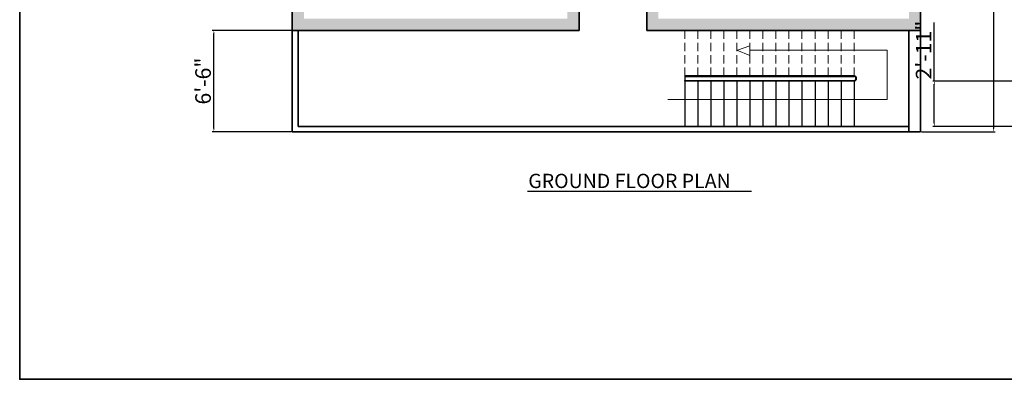
# Model space of a CAD drawing. Units: inches. Extents: x 1266 to 2869, y -408 to 3241.
# Tile 1 of 11: x 1266 to 2023, y 987 to 1264. Entities that reach past the tile are written whole.
import ezdxf

# ---------------------------------------------------------------- set-up
doc = ezdxf.new("R2010")
doc.units = ezdxf.units.IN
doc.linetypes.add('DASHED2', pattern=[9.525, 6.35, -3.175])
for name, color, linetype, lineweight in [('A-ANNO-DIMS', 2, 'Continuous', 18), ('A-ANNO-SYMB', 7, 'Continuous', 18), ('A-ANNO-TITL', 7, 'Continuous', 25), ('A-ANNO-TTLB', 7, 'Continuous', 35), ('A-FLOR-STRS', 7, 'Continuous', 25), ('A-FLOR-STRS-OVHD', 8, 'DASHED2', 18), ('A-WALL', 7, 'Continuous', 35), ('A-WALL-PATT', 251, 'Continuous', 13)]:
    doc.layers.add(name, color=color, linetype=linetype, lineweight=lineweight)
doc.styles.get("Standard").update_dxf_attribs({"font": 'arial.ttf'})
doc.dimstyles.new('ISO-25', dxfattribs={"dimtxt": 12, "dimasz": 2.5, "dimexe": 1.25, "dimexo": 0.625, "dimtad": 1, "dimdec": 0, "dimlunit": 3, "dimtxsty": 'Standard', "dimcen": 2.5, "dimadec": 0, "dimazin": 0, "dimtfac": 1, "dimtdec": 0, "dimtmove": 0, "dimatfit": 3, "dimfxl": 1, "dimarcsym": 0})

# ---------------------------------------------------------------- blocks, each defined once
blk = doc.blocks.new('*D3')
at = {"layer": 'A-ANNO-DIMS', "color": 0, "lineweight": -2, "transparency": 16777216}
for p, q in [((1959.32, 2278.35), (2016.1, 2278.35)), ((2014.85, 2275.85), (2014.85, 1179.85)), ((1959.32, 1177.35), (2016.1, 1177.35))]:
    blk.add_line(p, q, dxfattribs=at)
at = {"layer": 'A-ANNO-DIMS', "color": 0, "transparency": 16777216}
for points in [[(2014.43, 2275.85), (2015.27, 2275.85), (2014.85, 2278.35)], [(2014.43, 1179.85), (2015.27, 1179.85), (2014.85, 1177.35)]]:
    blk.add_solid(points, dxfattribs=at)
at = {"layer": 'Defpoints', "color": 0, "transparency": 16777216}
for p in [(1958.69, 2278.35), (1958.69, 1177.35), (2014.85, 1177.35)]:
    blk.add_point(p, dxfattribs=at)
at = {"layer": 'A-ANNO-DIMS', "color": 0, "transparency": 16777216, "insert": (2008.1, 1727.85), "char_height": 12, "attachment_point": 5, "rotation": 90}
blk.add_mtext('91\'-9"', dxfattribs=at)
blk = doc.blocks.new('STAIR-PATH-RETURN')
for p, q in [((53.2, 38.03), (63.2, 33.87)), ((53.5, 38.03), (53.2, 38.03)), ((63.2, 41.3), (53.5, 38.03)), ((63.2, 33.87), (63.2, 41.3)), ((168.66, 38.03), (63.2, 38.03)), ((168.66, 0), (168.66, 38.03)), ((0, 0), (168.66, 0))]:
    blk.add_line(p, q)
blk = doc.blocks.new('*D84')
at = {"layer": 'A-ANNO-DIMS', "color": 0, "lineweight": -2, "transparency": 16777216}
for p, q in [((1475.07, 1255.35), (1414.24, 1255.35)), ((1415.49, 1179.85), (1415.49, 1252.85)), ((1475.07, 1177.35), (1414.24, 1177.35))]:
    blk.add_line(p, q, dxfattribs=at)
at = {"layer": 'A-ANNO-DIMS', "color": 0, "transparency": 16777216}
for points in [[(1415.08, 1252.85), (1415.91, 1252.85), (1415.49, 1255.35)], [(1415.08, 1179.85), (1415.91, 1179.85), (1415.49, 1177.35)]]:
    blk.add_solid(points, dxfattribs=at)
at = {"layer": 'Defpoints', "color": 0, "transparency": 16777216}
for p in [(1415.49, 1255.35), (1475.69, 1255.35), (1475.69, 1177.35)]:
    blk.add_point(p, dxfattribs=at)
at = {"layer": 'A-ANNO-DIMS', "color": 0, "transparency": 16777216, "insert": (1408.74, 1216.35), "char_height": 12, "attachment_point": 5, "rotation": 90}
blk.add_mtext('6\'-6"', dxfattribs=at)
blk = doc.blocks.new('*D87')
at = {"layer": 'A-ANNO-DIMS', "color": 0, "lineweight": -2, "transparency": 16777216}
for p, q in [((1969.26, 1216.35), (1969.26, 1261.52)), ((2453.69, 1216.35), (1968.01, 1216.35)), ((1969.26, 1183.9), (1969.26, 1213.85)), ((2453.69, 1181.4), (1968.01, 1181.4))]:
    blk.add_line(p, q, dxfattribs=at)
at = {"layer": 'A-ANNO-DIMS', "color": 0, "transparency": 16777216}
for points in [[(1968.84, 1213.85), (1969.68, 1213.85), (1969.26, 1216.35)], [(1968.84, 1183.9), (1969.68, 1183.9), (1969.26, 1181.4)]]:
    blk.add_solid(points, dxfattribs=at)
at = {"layer": 'Defpoints', "color": 0, "transparency": 16777216}
for p in [(1969.26, 1216.35), (2454.31, 1216.35), (2454.31, 1181.4)]:
    blk.add_point(p, dxfattribs=at)
at = {"layer": 'A-ANNO-DIMS', "color": 0, "transparency": 16777216, "insert": (1962.61, 1240.19), "char_height": 12, "attachment_point": 5, "rotation": 90}
blk.add_mtext('2\'-11"', dxfattribs=at)

msp = doc.modelspace()

# ---------------------------------------------------------------- hatches: boundary and pattern name
at = {"layer": 'A-WALL-PATT'}
h = msp.add_hatch(color=256, dxfattribs=at)
h.dxf.hatch_style = 1
h.paths.add_polyline_path([(1484.69, 2269.35), (1562.69, 2269.35), (1562.69, 2149.35), (1558.42, 2149.35), (1558.42, 2144.85), (1567.19, 2144.85), (1573.23, 2144.85), (1573.23, 2146.74), (1573.23, 2149.35), (1567.19, 2149.35), (1567.19, 2269.35), (1597.45, 2269.35), (1597.45, 2273.85), (1597.45, 2278.35), (1475.69, 2278.35), (1475.69, 2234.52), (1484.69, 2234.52)])
h.paths.add_polyline_path([(1873.25, 2278.35), (1748.19, 2278.35), (1696.19, 2278.35), (1657.45, 2278.35), (1657.45, 2269.35), (1687.19, 2269.35), (1687.19, 2149.35), (1651.94, 2149.35), (1651.94, 2144.85), (1687.19, 2144.85), (1687.19, 2133.61), (1696.19, 2133.61), (1696.19, 2269.35), (1748.19, 2269.35), (1748.19, 2234.52), (1757.19, 2234.52), (1757.19, 2269.35), (1835.19, 2269.35), (1835.19, 2149.35), (1827.33, 2149.35), (1827.33, 2144.85), (1843.74, 2144.85), (1843.74, 2149.35), (1839.69, 2149.35), (1839.69, 2269.35), (1873.25, 2269.35), (1873.25, 2273.85)])
h.paths.add_polyline_path([(1958.69, 2278.35), (1933.25, 2278.35), (1933.25, 2269.35), (1949.69, 2269.35), (1949.69, 2149.35), (1912.22, 2149.35), (1912.22, 2144.85), (1949.69, 2144.85), (1949.69, 2133.61), (1958.69, 2133.61)])
h.paths.add_polyline_path([(1883.69, 2144.85), (1889.08, 2144.85), (1889.08, 2149.35), (1875.58, 2149.35), (1875.58, 2144.85), (1879.19, 2144.85), (1879.19, 2092.35), (1949.69, 2092.35), (1949.69, 2086.89), (1949.69, 2024.85), (1933.25, 2024.85), (1933.25, 2015.85), (1949.69, 2015.85), (1949.69, 1895.85), (1912.45, 1895.85), (1912.45, 1891.35), (1949.69, 1891.35), (1949.69, 1880.11), (1958.69, 1880.11), (1958.69, 2086.89), (1958.69, 2109.61), (1949.69, 2109.61), (1949.69, 2096.85), (1883.69, 2096.85)])
h.paths.add_polyline_path([(1757.19, 2198.52), (1748.19, 2198.52), (1748.19, 2086.89), (1757.19, 2086.89), (1757.19, 2144.85), (1793.55, 2144.85), (1793.55, 2149.35), (1757.19, 2149.35)])
h.paths.add_polyline_path([(1696.19, 2109.61), (1687.19, 2109.61), (1687.19, 2096.85), (1621.19, 2096.85), (1621.19, 2144.85), (1627.24, 2144.85), (1627.24, 2149.35), (1616.69, 2149.35), (1610.35, 2149.35), (1610.35, 2144.85), (1616.69, 2144.85), (1616.69, 2092.35), (1687.19, 2092.35), (1687.19, 2086.89), (1696.19, 2086.89)], flags=17)
h.paths.add_polyline_path([(1484.69, 2144.85), (1520.8, 2144.85), (1520.8, 2149.35), (1484.69, 2149.35), (1484.69, 2198.52), (1475.69, 2198.52), (1475.69, 1981.02), (1484.69, 1981.02), (1484.69, 2015.85), (1687.19, 2015.85), (1687.19, 1895.85), (1650.13, 1895.85), (1650.13, 1891.35), (1687.19, 1891.35), (1687.19, 1880.11), (1696.19, 1880.11), (1696.19, 2035.62), (1687.19, 2035.62), (1687.19, 2024.85), (1484.69, 2024.85)])
h.paths.add_polyline_path([(1484.69, 1691.52), (1475.69, 1691.52), (1475.69, 1474.02), (1484.69, 1474.02)])
h.paths.add_polyline_path([(1518.03, 1895.85), (1484.69, 1895.85), (1484.69, 1945.02), (1475.69, 1945.02), (1475.69, 1727.52), (1484.69, 1727.52), (1484.69, 1762.35), (1687.19, 1762.35), (1687.19, 1642.35), (1651.94, 1642.35), (1651.94, 1637.85), (1687.19, 1637.85), (1687.19, 1589.85), (1621.19, 1589.85), (1621.19, 1637.85), (1627.19, 1637.85), (1627.19, 1642.35), (1610.89, 1642.35), (1610.89, 1637.85), (1616.69, 1637.85), (1616.69, 1585.35), (1687.19, 1585.35), (1687.19, 1579.45), (1696.19, 1579.45), (1696.19, 1779.84), (1687.19, 1779.84), (1687.19, 1771.35), (1484.69, 1771.35), (1484.69, 1891.35), (1518.03, 1891.35)])
h.paths.add_polyline_path([(1567.19, 2015.85), (1562.69, 2015.85), (1562.69, 1895.85), (1555.64, 1895.85), (1555.64, 1891.35), (1570.46, 1891.35), (1570.46, 1895.85), (1567.19, 1895.85)], flags=17)
h.paths.add_polyline_path([(1625.43, 1895.85), (1607.58, 1895.85), (1607.58, 1891.35), (1616.69, 1891.35), (1616.69, 1838.85), (1687.19, 1838.85), (1687.19, 1831.11), (1696.19, 1831.11), (1696.19, 1856.11), (1687.19, 1856.11), (1687.19, 1843.35), (1621.19, 1843.35), (1621.19, 1891.35), (1625.43, 1891.35)], flags=17)
h.paths.add_polyline_path([(1567.19, 1762.35), (1562.69, 1762.35), (1562.69, 1642.35), (1558.42, 1642.35), (1558.42, 1637.85), (1573.23, 1637.85), (1573.23, 1642.35), (1567.19, 1642.35)], flags=17)
h.paths.add_polyline_path([(1520.8, 1642.35), (1484.69, 1642.35), (1484.69, 1637.85), (1520.8, 1637.85)], flags=17)
h.paths.add_polyline_path([(1687.19, 1517.85), (1484.69, 1517.85), (1484.69, 1508.85), (1562.69, 1508.85), (1562.69, 1388.85), (1567.19, 1388.85), (1567.19, 1508.85), (1687.19, 1508.85)])
h.paths.add_polyline_path([(1696.19, 1528.18), (1687.19, 1528.18), (1687.19, 1323.21), (1696.19, 1323.21)])
h.paths.add_polyline_path([(1696.19, 1271.94), (1687.19, 1271.94), (1687.19, 1264.35), (1484.69, 1264.35), (1484.69, 1283.77), (1480.19, 1283.77), (1475.69, 1283.77), (1475.69, 1255.35), (1480.19, 1255.35), (1696.19, 1255.35)])
h.paths.add_polyline_path([(1484.69, 1438.02), (1475.69, 1438.02), (1475.69, 1319.77), (1484.69, 1319.77)])
h.paths.add_polyline_path([(1873.25, 1513.35), (1873.25, 1517.85), (1757.19, 1517.85), (1757.19, 1528.62), (1748.19, 1528.62), (1748.19, 1474.02), (1757.19, 1474.02), (1757.19, 1508.85), (1835.19, 1508.85), (1835.19, 1388.85), (1827.33, 1388.85), (1827.33, 1384.35), (1843.74, 1384.35), (1843.74, 1388.85), (1839.69, 1388.85), (1839.69, 1508.85), (1873.25, 1508.85)])
h.paths.add_polyline_path([(1958.69, 1602.61), (1949.69, 1602.61), (1949.69, 1517.85), (1933.25, 1517.85), (1933.25, 1508.85), (1949.69, 1508.85), (1949.69, 1388.85), (1912.22, 1388.85), (1912.22, 1384.35), (1949.69, 1384.35), (1949.69, 1373.11), (1958.69, 1373.11)])
h.paths.add_polyline_path([(1958.69, 1349.11), (1949.69, 1349.11), (1949.69, 1336.35), (1883.69, 1336.35), (1883.69, 1384.35), (1889.08, 1384.35), (1889.08, 1388.85), (1875.58, 1388.85), (1875.58, 1384.35), (1879.19, 1384.35), (1879.19, 1331.85), (1949.69, 1331.85), (1949.69, 1315.59), (1958.69, 1315.59)])
h.paths.add_polyline_path([(1958.69, 1279.59), (1954.19, 1279.59), (1949.69, 1279.59), (1949.69, 1264.35), (1757.19, 1264.35), (1757.19, 1275.12), (1748.19, 1275.12), (1748.19, 1255.35), (1958.69, 1255.35)])
h.paths.add_polyline_path([(1757.19, 1438.02), (1748.19, 1438.02), (1748.19, 1326.39), (1757.19, 1326.39)])
h.paths.add_polyline_path([(1793.55, 1388.85), (1757.19, 1388.85), (1757.19, 1384.35), (1793.55, 1384.35)], flags=0)

# ---------------------------------------------------------------- linework, layer by layer
at = {"layer": 'A-ANNO-TITL'}
msp.add_line((1656.57, 1131.68), (1828.73, 1131.68), dxfattribs=at)
at = {"layer": 'A-ANNO-TTLB'}
msp.add_lwpolyline([(1266.23, 3241.34), (2868.62, 3241.34), (2868.62, 986.84), (1266.23, 986.84)], close=True, dxfattribs=at)
at = {"layer": 'A-FLOR-STRS'}
for p, q in [((1907.55, 1220.35), (1777.55, 1220.35)), ((1777.55, 1220.35), (1777.55, 1216.35)), ((1777.55, 1220.35), (1777.55, 1219.85)), ((1777.55, 1219.85), (1907.55, 1219.85)), ((1777.55, 1216.35), (1777.55, 1216.85)), ((1777.55, 1216.85), (1907.55, 1216.85)), ((1907.55, 1216.35), (1777.55, 1216.35)), ((1777.55, 1216.35), (1777.55, 1181.4)), ((1787.55, 1216.35), (1787.55, 1181.4)), ((1797.55, 1216.35), (1797.55, 1181.4)), ((1807.55, 1216.35), (1807.55, 1181.4)), ((1817.55, 1216.35), (1817.55, 1181.4)), ((1827.55, 1216.35), (1827.55, 1181.4)), ((1837.55, 1216.35), (1837.55, 1181.4)), ((1847.55, 1216.35), (1847.55, 1181.4)), ((1857.55, 1216.35), (1857.55, 1181.4)), ((1867.55, 1216.35), (1867.55, 1181.4)), ((1877.55, 1216.35), (1877.55, 1181.4)), ((1887.55, 1216.35), (1887.55, 1181.4)), ((1897.55, 1216.35), (1897.55, 1181.4)), ((1907.55, 1216.35), (1907.55, 1181.4))]:
    msp.add_line(p, q, dxfattribs=at)
for radius in [2, 1.5]:
    msp.add_arc((1907.55, 1218.35), radius, 270, 90, dxfattribs=at)
at = {"layer": 'A-FLOR-STRS-OVHD'}
for p, q in [((1777.55, 1220.35), (1777.55, 1255.35)), ((1787.55, 1220.35), (1787.55, 1255.35)), ((1797.55, 1220.35), (1797.55, 1255.35)), ((1807.55, 1220.35), (1807.55, 1255.35)), ((1817.55, 1220.35), (1817.55, 1255.35)), ((1827.55, 1220.35), (1827.55, 1255.35)), ((1837.55, 1220.35), (1837.55, 1255.35)), ((1847.55, 1220.35), (1847.55, 1255.35)), ((1857.55, 1220.35), (1857.55, 1255.35)), ((1867.55, 1220.35), (1867.55, 1255.35)), ((1877.55, 1220.35), (1877.55, 1255.35)), ((1887.55, 1220.35), (1887.55, 1255.35)), ((1897.55, 1220.35), (1897.55, 1255.35)), ((1907.55, 1220.35), (1907.55, 1255.35))]:
    msp.add_line(p, q, dxfattribs=at)
at = {"layer": 'A-WALL'}
for p, q in [((1475.69, 2278.35), (1475.69, 1255.35)), ((1958.69, 1255.35), (1958.69, 2086.89)), ((1696.19, 1271.94), (1696.19, 1255.35)), ((1748.19, 1275.12), (1748.19, 1255.35)), ((1475.69, 1255.35), (1696.19, 1255.35)), ((1475.69, 1255.35), (1475.69, 1177.35)), ((1475.69, 1255.35), (1480.19, 1255.35)), ((1480.19, 1255.35), (1480.19, 1181.4)), ((1748.19, 1255.35), (1958.69, 1255.35)), ((1949.69, 1255.35), (1949.69, 1177.35)), ((1949.69, 1255.35), (1949.69, 1218.35)), ((1958.69, 1255.35), (1958.69, 1177.35)), ((1480.19, 1181.4), (1949.69, 1181.4)), ((1475.69, 1177.35), (1748.19, 1177.35)), ((1748.19, 1177.35), (1958.69, 1177.35))]:
    msp.add_line(p, q, dxfattribs=at)

# ---------------------------------------------------------------- block references
at = {"layer": 'A-ANNO-SYMB'}
msp.add_blockref('STAIR-PATH-RETURN', (1764.36, 1202.19), dxfattribs=at)

# ---------------------------------------------------------------- texts
at = {"layer": 'A-ANNO-TITL', "insert": (1657.17, 1145), "char_height": 11, "attachment_point": 1}
msp.add_mtext_dynamic_manual_height_columns('GROUND FLOOR PLAN', width=423.8424, gutter_width=12.5, heights=[0], dxfattribs=at)

# ---------------------------------------------------------------- dimensions: what is measured, and where the dimension line sits
at = {"layer": 'A-ANNO-DIMS'}
for base, p1, p2, override, picture, middle in [((2014.85, 1177.35), (1958.69, 2278.35), (1958.69, 1177.35), {"dimclrd": 0, "dimclre": 0, "dimclrt": 0}, '*D3', (2008.1, 1727.85)), ((1969.2585, 1216.3471), (2454.3125, 1181.4021), (2454.3125, 1216.3471), {"dimdec": 1, "dimlfac": 1, "dimrnd": 0, "dimzin": 1, "dimdsep": 46, "dimlunit": 4, "dimfrac": 2}, '*D87', (1962.609, 1240.1856)), ((1415.49, 1255.35), (1475.69, 1177.35), (1475.69, 1255.35), {"dimdec": 1, "dimlfac": 1, "dimrnd": 0, "dimzin": 1, "dimdsep": 46, "dimlunit": 4, "dimfrac": 2}, '*D84', (1408.74, 1216.35))]:
    dim = msp.add_linear_dim(base=base, p1=p1, p2=p2, angle=90, dimstyle='ISO-25', override=override, dxfattribs=at)
    dim.commit()
    dim.dimension.update_dxf_attribs({"geometry": picture, "text_midpoint": middle})

doc.saveas('drawing.dxf')
